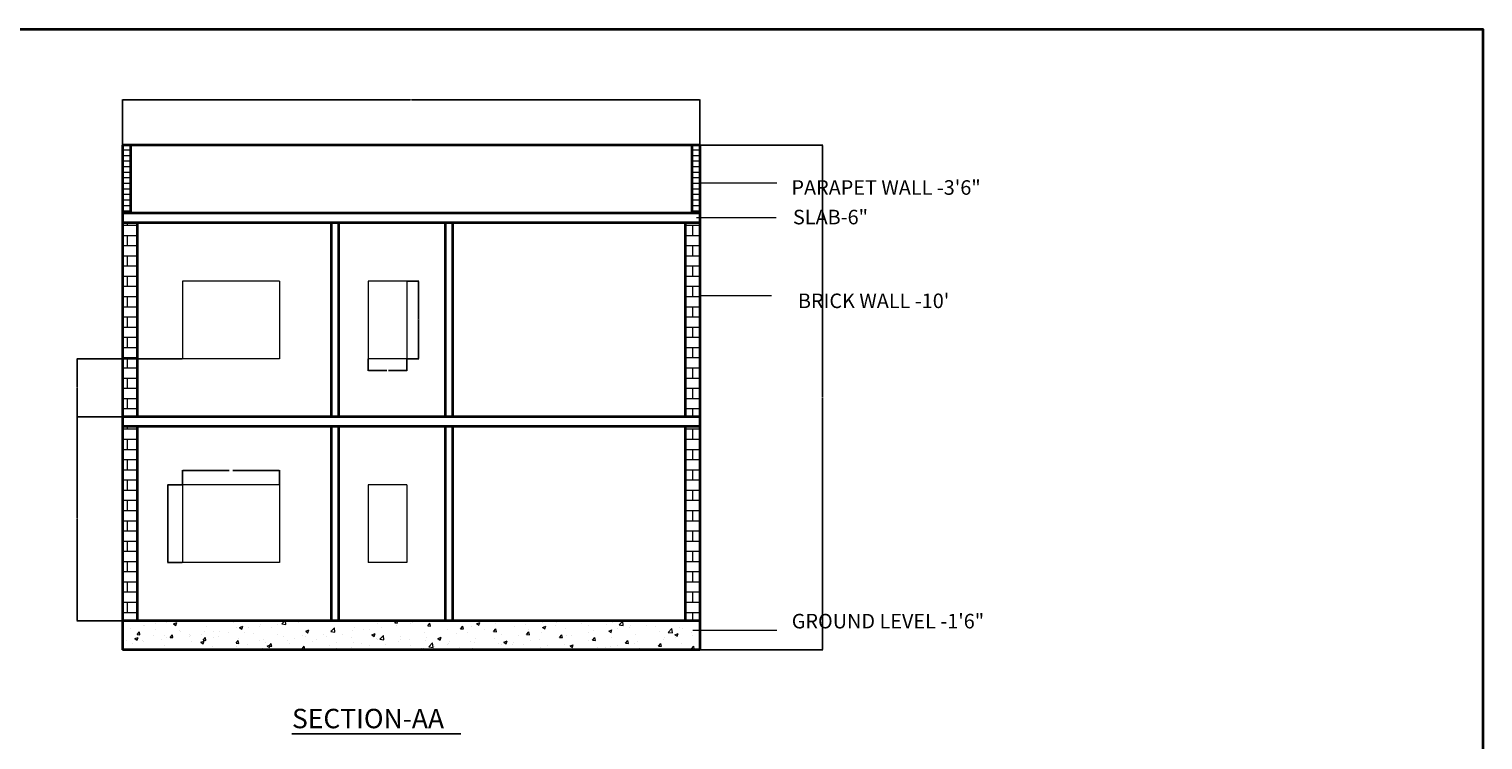
# Model space of a CAD drawing. Units: inches. Extents: x 1912 to 3731, y 1384 to 2459.
# Tile 8 of 8: x 2821 to 3720, y 2019 to 2459. Entities that reach past the tile are written whole.
import ezdxf

# ---------------------------------------------------------------- set-up
doc = ezdxf.new("R2010")
doc.units = ezdxf.units.IN
for name, color, linetype, lineweight in [('A-ANNO-DIMS', 2, 'Continuous', 18), ('A-ANNO-TEXT', 7, 'Continuous', 18), ('A-ANNO-TITL', 7, 'Continuous', 25), ('A-ANNO-TTLB', 7, 'Continuous', 35), ('A-GLAZ', 4, 'Continuous', 18), ('A-SECT', 7, 'Continuous', 35), ('A-WALL-PATT', 252, 'Continuous', 13), ('S-SLAB', 7, 'Continuous', 35), ('S-SLAB-PATT', 252, 'Continuous', 13)]:
    doc.layers.add(name, color=color, linetype=linetype, lineweight=lineweight)
doc.styles.get("Standard").update_dxf_attribs({"font": 'arial.ttf'})
doc.dimstyles.get("Standard").update_dxf_attribs({"dimtxt": 0.18, "dimasz": 0.18, "dimexe": 0.18, "dimexo": 0.0625, "dimgap": 0.09, "dimtad": 0, "dimtih": 1, "dimtoh": 1, "dimdec": 4, "dimzin": 0, "dimdsep": 46, "dimtxsty": 'Standard', "dimcen": 0.09, "dimadec": 0, "dimazin": 0, "dimtfac": 1, "dimtdec": 4, "dimtofl": 0, "dimtmove": 0, "dimatfit": 3, "dimfxl": 1, "dimtolj": 1, "dimtzin": 0, "dimarcsym": 0})

# ---------------------------------------------------------------- blocks, each defined once
blk = doc.blocks.new('WIN-SECTION-60X48')
for p, q in [((0, 48), (0, 0)), ((60, 48), (0, 48)), ((60, 48), (60, 0)), ((60, 0), (0, 0))]:
    blk.add_line(p, q)
blk = doc.blocks.new('WIN-SECTION-24X48')
for p, q in [((0, 48), (0, 0)), ((24, 48), (0, 48)), ((24, 48), (24, 0)), ((24, 0), (0, 0))]:
    blk.add_line(p, q)
blk = doc.blocks.new('*D43')
at = {"layer": 'A-ANNO-DIMS', "color": 0, "lineweight": -2, "transparency": 16777216}
for p, q in [((2915.82, 2176.8), (2915.82, 2185.91)), ((2916, 2185.73), (2944.7, 2185.73)), ((2975.64, 2185.73), (2946.94, 2185.73)), ((2975.82, 2176.8), (2975.82, 2185.91))]:
    blk.add_line(p, q, dxfattribs=at)
at = {"layer": 'A-ANNO-DIMS', "color": 0, "transparency": 16777216}
for points in [[(2916, 2185.76), (2916, 2185.7), (2915.82, 2185.73)], [(2975.64, 2185.76), (2975.64, 2185.7), (2975.82, 2185.73)]]:
    blk.add_solid(points, dxfattribs=at)
at = {"layer": 'Defpoints', "color": 0, "transparency": 16777216}
for p in [(2975.82, 2185.73), (2915.82, 2176.73), (2975.82, 2176.73)]:
    blk.add_point(p, dxfattribs=at)
at = {"layer": 'A-ANNO-DIMS', "color": 0, "transparency": 16777216, "insert": (2945.82, 2185.73), "char_height": 0.18, "attachment_point": 5}
blk.add_mtext('\\A1;WINDOW 60 TYP.', dxfattribs=at)
blk = doc.blocks.new('*D44')
at = {"layer": 'A-ANNO-DIMS', "color": 0, "lineweight": -2, "transparency": 16777216}
for p, q in [((2915.75, 2176.73), (2906.64, 2176.73)), ((2906.82, 2176.55), (2906.82, 2152.92)), ((2906.82, 2128.91), (2906.82, 2152.55)), ((2915.75, 2128.73), (2906.64, 2128.73))]:
    blk.add_line(p, q, dxfattribs=at)
at = {"layer": 'A-ANNO-DIMS', "color": 0, "transparency": 16777216}
for points in [[(2906.79, 2176.55), (2906.85, 2176.55), (2906.82, 2176.73)], [(2906.79, 2128.91), (2906.85, 2128.91), (2906.82, 2128.73)]]:
    blk.add_solid(points, dxfattribs=at)
at = {"layer": 'Defpoints', "color": 0, "transparency": 16777216}
for p in [(2906.82, 2176.73), (2915.82, 2176.73), (2915.82, 2128.73)]:
    blk.add_point(p, dxfattribs=at)
at = {"layer": 'A-ANNO-DIMS', "color": 0, "transparency": 16777216, "insert": (2906.82, 2152.73), "char_height": 0.18, "attachment_point": 5}
blk.add_mtext('\\A1;48 TYP.', dxfattribs=at)
blk = doc.blocks.new('*D45')
at = {"layer": 'A-ANNO-DIMS', "color": 0, "lineweight": -2, "transparency": 16777216}
for p, q in [((3054.8, 2302.73), (3062.12, 2302.73)), ((3061.94, 2302.55), (3061.94, 2278.92)), ((3061.94, 2254.91), (3061.94, 2278.55)), ((3054.8, 2254.73), (3062.12, 2254.73))]:
    blk.add_line(p, q, dxfattribs=at)
at = {"layer": 'A-ANNO-DIMS', "color": 0, "transparency": 16777216}
for points in [[(3061.91, 2302.55), (3061.97, 2302.55), (3061.94, 2302.73)], [(3061.91, 2254.91), (3061.97, 2254.91), (3061.94, 2254.73)]]:
    blk.add_solid(points, dxfattribs=at)
at = {"layer": 'Defpoints', "color": 0, "transparency": 16777216}
for p in [(3054.74, 2302.73), (3061.94, 2302.73), (3054.74, 2254.73)]:
    blk.add_point(p, dxfattribs=at)
at = {"layer": 'A-ANNO-DIMS', "color": 0, "transparency": 16777216, "insert": (3061.94, 2278.73), "char_height": 0.18, "attachment_point": 5}
blk.add_mtext('\\A1;WINDOW 48 TYP.', dxfattribs=at)
blk = doc.blocks.new('*D46')
at = {"layer": 'A-ANNO-DIMS', "color": 0, "lineweight": -2, "transparency": 16777216}
for p, q in [((3030.74, 2254.67), (3030.74, 2247.35)), ((3054.74, 2254.67), (3054.74, 2247.35)), ((3030.92, 2247.53), (3042.21, 2247.53)), ((3054.56, 2247.53), (3043.27, 2247.53))]:
    blk.add_line(p, q, dxfattribs=at)
at = {"layer": 'A-ANNO-DIMS', "color": 0, "transparency": 16777216}
for points in [[(3030.92, 2247.56), (3030.92, 2247.5), (3030.74, 2247.53)], [(3054.56, 2247.56), (3054.56, 2247.5), (3054.74, 2247.53)]]:
    blk.add_solid(points, dxfattribs=at)
at = {"layer": 'Defpoints', "color": 0, "transparency": 16777216}
for p in [(3030.74, 2254.73), (3054.74, 2254.73), (3054.74, 2247.53)]:
    blk.add_point(p, dxfattribs=at)
at = {"layer": 'A-ANNO-DIMS', "color": 0, "transparency": 16777216, "insert": (3042.74, 2247.53), "char_height": 0.18, "attachment_point": 5}
blk.add_mtext('\\A1;24 TYP.', dxfattribs=at)
blk = doc.blocks.new('*D123')
at = {"layer": 'A-ANNO-DIMS', "color": 0, "lineweight": -2, "transparency": 16777216}
for p, q in [((2878.79, 2386.8), (2878.79, 2415.06)), ((2878.97, 2414.88), (3057, 2414.88)), ((3235.61, 2414.88), (3057.57, 2414.88)), ((3235.79, 2386.8), (3235.79, 2415.06))]:
    blk.add_line(p, q, dxfattribs=at)
at = {"layer": 'A-ANNO-DIMS', "color": 0, "transparency": 16777216}
for points in [[(2878.97, 2414.91), (2878.97, 2414.85), (2878.79, 2414.88)], [(3235.61, 2414.91), (3235.61, 2414.85), (3235.79, 2414.88)]]:
    blk.add_solid(points, dxfattribs=at)
at = {"layer": 'Defpoints', "color": 0, "transparency": 16777216}
for p in [(3235.79, 2414.88), (2878.79, 2386.73), (3235.79, 2386.73)]:
    blk.add_point(p, dxfattribs=at)
at = {"layer": 'A-ANNO-DIMS', "color": 0, "transparency": 16777216, "insert": (3057.29, 2414.88), "char_height": 0.18, "attachment_point": 5}
blk.add_mtext('\\A1;357', dxfattribs=at)
blk = doc.blocks.new('*D124')
at = {"layer": 'A-ANNO-DIMS', "color": 0, "lineweight": -2, "transparency": 16777216}
for p, q in [((3235.85, 2386.73), (3311.89, 2386.73)), ((3311.71, 2386.55), (3311.71, 2230.92)), ((3311.71, 2074.91), (3311.71, 2230.55)), ((3235.85, 2074.73), (3311.89, 2074.73))]:
    blk.add_line(p, q, dxfattribs=at)
at = {"layer": 'A-ANNO-DIMS', "color": 0, "transparency": 16777216}
for points in [[(3311.68, 2386.55), (3311.74, 2386.55), (3311.71, 2386.73)], [(3311.68, 2074.91), (3311.74, 2074.91), (3311.71, 2074.73)]]:
    blk.add_solid(points, dxfattribs=at)
at = {"layer": 'Defpoints', "color": 0, "transparency": 16777216}
for p in [(3235.79, 2386.73), (3311.71, 2386.73), (3235.79, 2074.73)]:
    blk.add_point(p, dxfattribs=at)
at = {"layer": 'A-ANNO-DIMS', "color": 0, "transparency": 16777216, "insert": (3311.71, 2230.73), "char_height": 0.18, "attachment_point": 5}
blk.add_mtext('\\A1;312', dxfattribs=at)
blk = doc.blocks.new('*D125')
at = {"layer": 'A-ANNO-DIMS', "color": 0, "lineweight": -2, "transparency": 16777216}
for p, q in [((2878.72, 2218.73), (2850.46, 2218.73)), ((2850.64, 2218.55), (2850.64, 2155.92)), ((2850.64, 2092.91), (2850.64, 2155.55)), ((2878.72, 2092.73), (2850.46, 2092.73))]:
    blk.add_line(p, q, dxfattribs=at)
at = {"layer": 'A-ANNO-DIMS', "color": 0, "transparency": 16777216}
for points in [[(2850.61, 2218.55), (2850.67, 2218.55), (2850.64, 2218.73)], [(2850.61, 2092.91), (2850.67, 2092.91), (2850.64, 2092.73)]]:
    blk.add_solid(points, dxfattribs=at)
at = {"layer": 'Defpoints', "color": 0, "transparency": 16777216}
for p in [(2850.64, 2218.73), (2878.79, 2218.73), (2878.79, 2092.73)]:
    blk.add_point(p, dxfattribs=at)
at = {"layer": 'A-ANNO-DIMS', "color": 0, "transparency": 16777216, "insert": (2850.64, 2155.73), "char_height": 0.18, "attachment_point": 5}
blk.add_mtext('\\A1;126', dxfattribs=at)
blk = doc.blocks.new('*D126')
at = {"layer": 'A-ANNO-DIMS', "color": 0, "lineweight": -2, "transparency": 16777216}
for p, q in [((2915.75, 2254.73), (2850.46, 2254.73)), ((2850.64, 2254.55), (2850.64, 2236.92)), ((2850.64, 2218.91), (2850.64, 2236.55)), ((2878.72, 2218.73), (2850.46, 2218.73))]:
    blk.add_line(p, q, dxfattribs=at)
at = {"layer": 'A-ANNO-DIMS', "color": 0, "transparency": 16777216}
for points in [[(2850.61, 2254.55), (2850.67, 2254.55), (2850.64, 2254.73)], [(2850.61, 2218.91), (2850.67, 2218.91), (2850.64, 2218.73)]]:
    blk.add_solid(points, dxfattribs=at)
at = {"layer": 'Defpoints', "color": 0, "transparency": 16777216}
for p in [(2850.64, 2254.73), (2915.82, 2254.73), (2878.79, 2218.73)]:
    blk.add_point(p, dxfattribs=at)
at = {"layer": 'A-ANNO-DIMS', "color": 0, "transparency": 16777216, "insert": (2850.64, 2236.73), "char_height": 0.18, "attachment_point": 5}
blk.add_mtext('\\A1;36', dxfattribs=at)

msp = doc.modelspace()

# ---------------------------------------------------------------- hatches: boundary and pattern name
at = {"layer": 'A-WALL-PATT'}
h = msp.add_hatch(dxfattribs=at)
h.set_pattern_fill('LINE', color=256, scale=1.080315, style=0)
h.paths.add_polyline_path([(2878.7856, 2344.7342), (2883.8549, 2344.7342), (2883.8549, 2386.7342), (2878.7856, 2386.7342)])
h = msp.add_hatch(dxfattribs=at)
h.set_pattern_fill('LINE', color=256, scale=1.080315, style=0)
h.paths.add_polyline_path([(3231.1484, 2344.7342), (3235.7856, 2344.7342), (3235.7856, 2386.7342), (3231.1484, 2386.7342)])
h = msp.add_hatch(dxfattribs=at)
h.set_pattern_fill('AR-BRSTD', color=256, scale=0.0930002, style=0)
h.paths.add_polyline_path([(2878.7856, 2218.7342), (2887.7856, 2218.7342), (2887.7856, 2338.7342), (2878.7856, 2338.7342)])
h = msp.add_hatch(dxfattribs=at)
h.set_pattern_fill('AR-BRSTD', color=256, scale=0.0930002, style=0)
h.paths.add_polyline_path([(3226.7856, 2218.7342), (3235.7856, 2218.7342), (3235.7856, 2338.7342), (3226.7856, 2338.7342)])
h = msp.add_hatch(dxfattribs=at)
h.set_pattern_fill('AR-BRSTD', color=256, scale=0.0930002, style=0)
h.paths.add_polyline_path([(2878.7856, 2092.7342), (2887.7856, 2092.7342), (2887.7856, 2212.7342), (2878.7856, 2212.7342)])
h = msp.add_hatch(dxfattribs=at)
h.set_pattern_fill('AR-BRSTD', color=256, scale=0.0930002, style=0)
h.paths.add_polyline_path([(3226.7856, 2092.7342), (3235.7856, 2092.7342), (3235.7856, 2212.7342), (3226.7856, 2212.7342)])
at = {"layer": 'S-SLAB-PATT'}
h = msp.add_hatch(dxfattribs=at)
h.set_pattern_fill('AR-CONC', color=256, scale=0.112, style=0)
h.paths.add_polyline_path([(2878.7856, 2074.7342), (3235.7856, 2074.7342), (3235.7856, 2092.7342), (2878.7856, 2092.7342)])

# ---------------------------------------------------------------- linework, layer by layer
at = {"layer": 'A-ANNO-TEXT'}
for p, q in [((3235.7856, 2363.4664), (3283.5634, 2363.4664)), ((3233.8538, 2342.0711), (3283.0977, 2342.0711)), ((3235.7856, 2293.7342), (3280.2871, 2293.7342)), ((3231.4426, 2086.9074), (3283.5034, 2086.9074))]:
    msp.add_line(p, q, dxfattribs=at)
at = {"layer": 'A-ANNO-TITL'}
msp.add_line((2983.5998, 2022.8419), (3088.1165, 2022.8419), dxfattribs=at)
at = {"layer": 'A-ANNO-TTLB'}
msp.add_lwpolyline([(1912.2029, 2458.5537), (3720.218, 2458.5537), (3720.218, 1383.9599), (1912.2029, 1383.9599)], close=True, dxfattribs=at)
at = {"layer": 'A-SECT'}
for p, q in [((2878.7856, 2386.7342), (2878.7856, 2200.7342)), ((3235.7856, 2386.7342), (2878.7856, 2386.7342)), ((2883.8549, 2344.7342), (2883.8549, 2386.7342)), ((3231.1484, 2344.7342), (3231.1484, 2386.7342)), ((3235.7856, 2386.7342), (3235.7856, 2200.7342)), ((2887.7856, 2338.7342), (2887.7856, 2218.7342)), ((3007.7856, 2338.7342), (3007.7856, 2218.7342)), ((3012.2856, 2338.7342), (3012.2856, 2218.7342)), ((3078.2856, 2338.7342), (3078.2856, 2218.7342)), ((3082.7856, 2338.7342), (3082.7856, 2218.7342)), ((3226.7856, 2338.7342), (3226.7856, 2218.7342)), ((2878.7856, 2260.7342), (2878.7856, 2074.7342)), ((3235.7856, 2260.7342), (3235.7856, 2074.7342)), ((2887.7856, 2212.7342), (2887.7856, 2092.7342)), ((3007.7856, 2212.7342), (3007.7856, 2092.7342)), ((3012.2856, 2212.7342), (3012.2856, 2092.7342)), ((3078.2856, 2212.7342), (3078.2856, 2092.7342)), ((3082.7856, 2212.7342), (3082.7856, 2092.7342)), ((3226.7856, 2212.7342), (3226.7856, 2092.7342))]:
    msp.add_line(p, q, dxfattribs=at)
at = {"layer": 'S-SLAB'}
for p, q in [((3235.7856, 2344.7342), (2878.7856, 2344.7342)), ((3235.7856, 2338.7342), (2878.7856, 2338.7342)), ((3235.7856, 2218.7342), (2878.7856, 2218.7342)), ((3235.7856, 2212.7342), (2878.7856, 2212.7342)), ((3235.7856, 2092.7342), (2878.7856, 2092.7342)), ((3235.7856, 2074.7342), (2878.7856, 2074.7342))]:
    msp.add_line(p, q, dxfattribs=at)

# ---------------------------------------------------------------- block references
at = {"layer": 'A-GLAZ'}
for name, p in [('WIN-SECTION-60X48', (2915.817, 2254.734)), ('WIN-SECTION-24X48', (3030.742, 2254.734)), ('WIN-SECTION-60X48', (2915.817, 2128.734)), ('WIN-SECTION-24X48', (3030.742, 2128.734))]:
    msp.add_blockref(name, p, dxfattribs=at)

# ---------------------------------------------------------------- texts
at = {"layer": 'A-ANNO-TEXT', "char_height": 9, "attachment_point": 1}
for s, width, insert in [('PARAPET WALL -3\'6"', 343.81547, (3292.5313, 2365.1126)), ('SLAB-6" ', 78.456729, (3293.4706, 2346.8351)), ("BRICK WALL -10'", 106.414239, (3296.5444, 2295.0399)), ('GROUND LEVEL -1\'6"', 169.163925, (3292.6993, 2096.9891))]:
    msp.add_mtext_dynamic_manual_height_columns(s, width=width, gutter_width=12.5, heights=[0], dxfattribs=dict(at, insert=insert))
at = {"layer": 'A-ANNO-TITL', "insert": (2983.6306, 2038.2635), "char_height": 12, "attachment_point": 1}
msp.add_mtext_dynamic_manual_height_columns('SECTION-AA', width=207.222429, gutter_width=12.5, heights=[0], dxfattribs=at)

# ---------------------------------------------------------------- dimensions: what is measured, and where the dimension line sits
at = {"layer": 'A-ANNO-DIMS'}
dim = msp.add_linear_dim(base=(3235.7856, 2414.8842), p1=(2878.7856, 2386.7342), p2=(3235.7856, 2386.7342), dimstyle='Standard', override={"dimdec": 0, "dimlfac": 1, "dimrnd": 0, "dimzin": 0, "dimdsep": 46, "dimlunit": 2}, dxfattribs=at)
dim.commit()
dim.dimension.update_dxf_attribs({"geometry": '*D123', "text_midpoint": (3057.2856, 2414.8842)})
for base, p1, p2, picture, middle in [((3311.7134, 2386.7342), (3235.7856, 2074.7342), (3235.7856, 2386.7342), '*D124', (3311.7134, 2230.7342)), ((2850.6356, 2254.7342), (2878.7856, 2218.7342), (2915.8175, 2254.7342), '*D126', (2850.6356, 2236.7342)), ((2850.6356, 2218.7342), (2878.7856, 2092.7342), (2878.7856, 2218.7342), '*D125', (2850.6356, 2155.7342))]:
    dim = msp.add_linear_dim(base=base, p1=p1, p2=p2, angle=90, dimstyle='Standard', override={"dimdec": 0, "dimlfac": 1, "dimrnd": 0, "dimzin": 0, "dimdsep": 46, "dimlunit": 2}, dxfattribs=at)
    dim.commit()
    dim.dimension.update_dxf_attribs({"geometry": picture, "text_midpoint": middle})
for base, p1, p2, text, picture, middle in [((3061.942, 2302.7342), (3054.742, 2254.7342), (3054.742, 2302.7342), 'WINDOW <> TYP.', '*D45', (3061.942, 2278.7342)), ((2906.8175, 2176.7342), (2915.8175, 2128.7342), (2915.8175, 2176.7342), '<> TYP.', '*D44', (2906.8175, 2152.7342))]:
    dim = msp.add_linear_dim(base=base, p1=p1, p2=p2, angle=90, text=text, dimstyle='Standard', override={"dimdec": 0, "dimlfac": 1, "dimrnd": 0, "dimzin": 0, "dimdsep": 46, "dimlunit": 2}, dxfattribs=at)
    dim.commit()
    dim.dimension.update_dxf_attribs({"geometry": picture, "text_midpoint": middle})
for base, p1, p2, text, picture, middle in [((3054.742, 2247.5342), (3030.742, 2254.7342), (3054.742, 2254.7342), '<> TYP.', '*D46', (3042.742, 2247.5342)), ((2975.8175, 2185.7342), (2915.8175, 2176.7342), (2975.8175, 2176.7342), 'WINDOW <> TYP.', '*D43', (2945.8175, 2185.7342))]:
    dim = msp.add_linear_dim(base=base, p1=p1, p2=p2, text=text, dimstyle='Standard', override={"dimdec": 0, "dimlfac": 1, "dimrnd": 0, "dimzin": 0, "dimdsep": 46, "dimlunit": 2}, dxfattribs=at)
    dim.commit()
    dim.dimension.update_dxf_attribs({"geometry": picture, "text_midpoint": middle})

doc.saveas('drawing.dxf')
